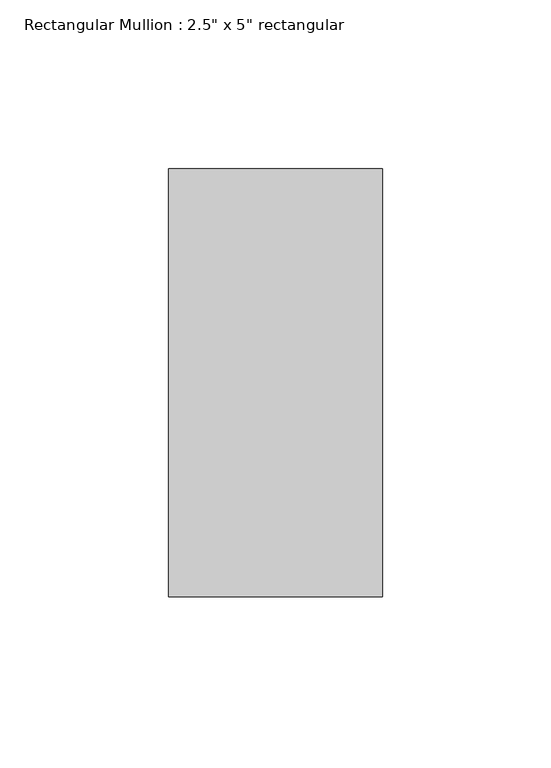
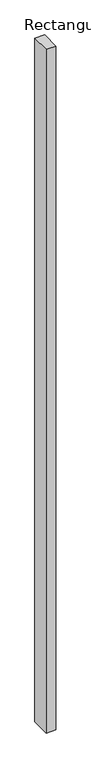
"""IFC4 building model written with IfcOpenShell, lengths in millimetres: member geometry."""

from ifc_helpers import new_model, si_unit, frame, origin, place, context, project, spatial, polyline, outline, extrude, source, transform, mapped, element, save


def member_3d8465bd(model_context):
    return source(origin(), model_context, "Body", "SweptSolid", [
        extrude(outline(polyline([(0.0, 63.5), (0.0, -63.5), (-63.5, -63.5), (-63.5, 63.5), (0.0, 63.5)])), frame((0.0, 0.0, -4743.0687315), z_axis=(0.0, 0.0, 1.0), x_axis=(1.0, 0.0, 0.0)), (0.0, 0.0, 1.0), 4743.0687315),
    ])


if __name__ == "__main__":
    model = new_model("IFC4")
    model_context = context("Model", 3, world=origin())
    ifc_project = project(units=[si_unit("LENGTHUNIT", "METRE", prefix="MILLI")], contexts=[model_context])
    site = spatial("IfcSite", under=ifc_project)
    building = spatial("IfcBuilding", under=site)
    placement = place(None, origin())
    member_shape = member_3d8465bd(model_context)
    element("IfcMember", 1, ObjectType="Rectangular Mullion : 2.5\" x 5\" rectangular", at=placement, inside=building, context=model_context, shape_type="MappedRepresentation", body=[
        mapped(member_shape, transform((0.0, 0.0, 0.0), x_axis=(1.0, 0.0, 0.0), y_axis=(0.0, 1.0, 0.0), z_axis=(0.0, 0.0, 1.0))),
    ])
    save(model, "model.ifc")

# Revit data of these elements
# Type "Rectangular Mullion : 2.5\" x 5\" rectangular"
#   built-in parameter 1007304 = 0.416667 (stored number, unit not read)
#   built-in parameter 1007301 = 0.104167 (stored number, unit not read)
#   built-in parameter 1007300 = 0.104167 (stored number, unit not read)
# Element 1 (IfcMember, "Rectangular Mullion : 2.5\" x 5\" rectangular")
#   Materials on its faces: "Aluminum"
# Materials
#   "Aluminum": class "Metal", colour RGB 247 247 247, transparency 0, Description = "Aluminum 6061", Cost = 0
